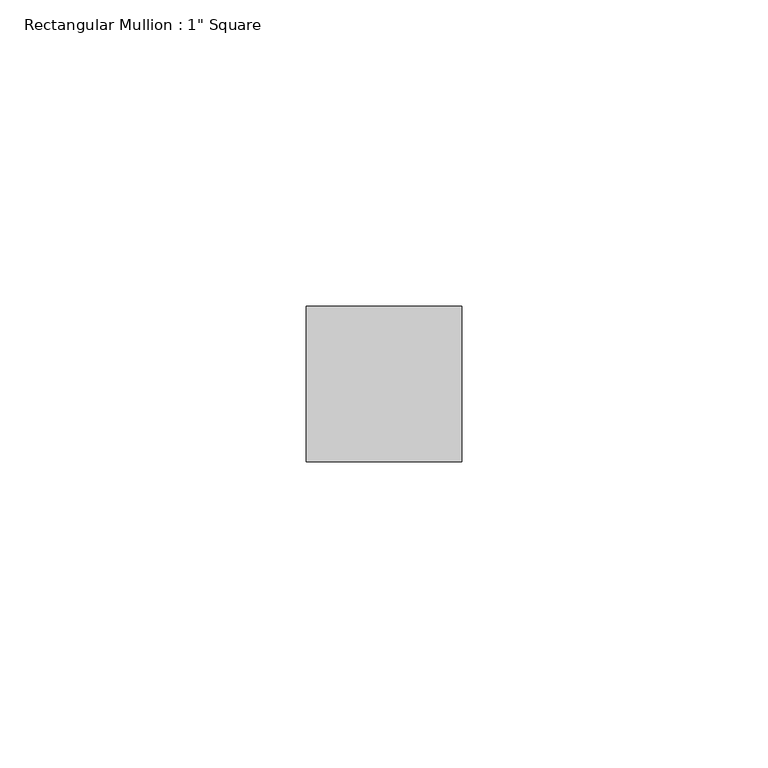
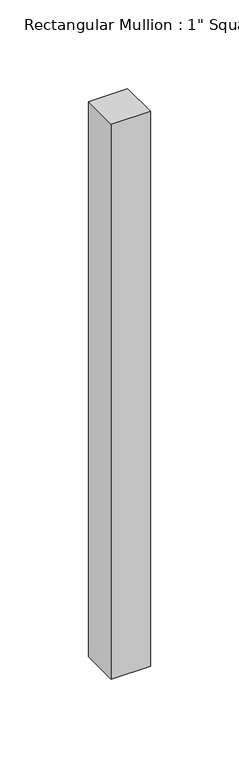
"""IFC4 building model written with IfcOpenShell, lengths in millimetres: member geometry."""

from ifc_helpers import new_model, si_unit, frame, origin, place, context, project, spatial, polyline, outline, extrude, source, transform, mapped, element, save


def member_b1407fb7(model_context):
    return source(origin(), model_context, "Body", "SweptSolid", [
        extrude(outline(polyline([(0.0, 12.7), (0.0, -12.7), (-25.4, -12.7), (-25.4, 12.7), (0.0, 12.7)])), frame((0.0, 0.0, -381.0), z_axis=(0.0, 0.0, 1.0), x_axis=(1.0, 0.0, 0.0)), (0.0, 0.0, 1.0), 381.0),
    ])


if __name__ == "__main__":
    model = new_model("IFC4")
    model_context = context("Model", 3, world=origin())
    ifc_project = project(units=[si_unit("LENGTHUNIT", "METRE", prefix="MILLI")], contexts=[model_context])
    site = spatial("IfcSite", under=ifc_project)
    building = spatial("IfcBuilding", under=site)
    placement = place(None, origin())
    member_shape = member_b1407fb7(model_context)
    element("IfcMember", 1, ObjectType="Rectangular Mullion : 1\" Square", at=placement, inside=building, context=model_context, shape_type="MappedRepresentation", body=[
        mapped(member_shape, transform((0.0, 0.0, 0.0), x_axis=(1.0, 0.0, 0.0), y_axis=(0.0, 1.0, 0.0), z_axis=(0.0, 0.0, 1.0))),
    ])
    save(model, "model.ifc")

# Revit data of these elements
# Type "Rectangular Mullion : 1\" Square"
#   built-in parameter 1007304 = 0.0833333 (stored number, unit not read)
#   built-in parameter 1007301 = 0.0416667 (stored number, unit not read)
#   built-in parameter 1007300 = 0.0416667 (stored number, unit not read)
